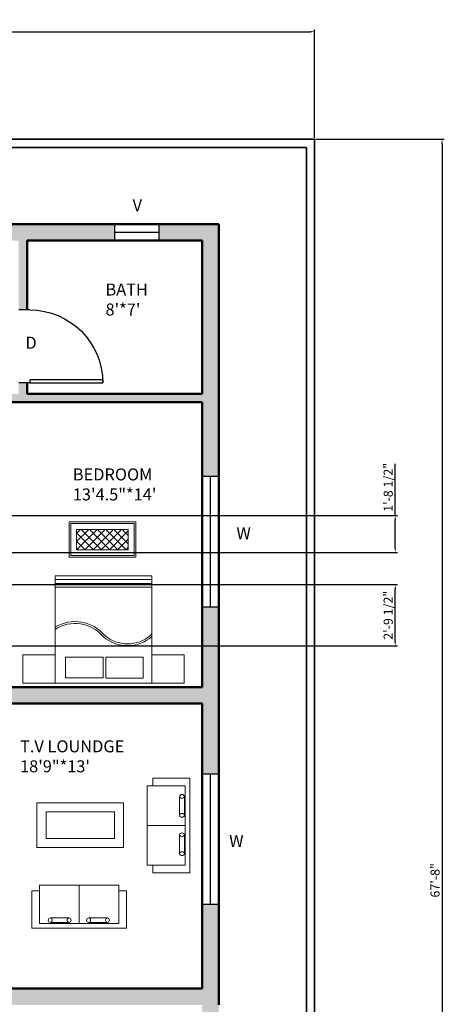
# Model space of a CAD drawing. Units: inches. Extents: x 2101 to 2663, y 1144 to 2069.
# Tile 4 of 4: x 2431 to 2663, y 1530 to 2069. Entities that reach past the tile are written whole.
import ezdxf

# ---------------------------------------------------------------- set-up
doc = ezdxf.new("R2010")
doc.units = ezdxf.units.IN
for name, color, linetype, lineweight in [('A-ANNO-DIMS', 2, 'Continuous', 18), ('A-ANNO-TEXT', 7, 'Continuous', 18), ('A-AREA-IDEN', 7, 'Continuous', 25), ('A-WALL-PATT', 240, 'Continuous', 13), ('C-PROP', 7, 'Continuous', 35), ('door', 52, 'Continuous', 25), ('fur', 142, 'Continuous', 18), ('wall', 240, 'Continuous', 50), ('win', 150, 'Continuous', 25)]:
    doc.layers.add(name, color=color, linetype=linetype, lineweight=lineweight)
doc.styles.get("Standard").update_dxf_attribs({"font": 'arial.ttf'})
doc.dimstyles.new('ISO-25', dxfattribs={"dimtxt": 5, "dimasz": 2.5, "dimexe": 1.25, "dimexo": 0.625, "dimtad": 1, "dimdec": 0, "dimlunit": 4, "dimtxsty": 'Standard', "dimcen": 2.5, "dimadec": 0, "dimazin": 0, "dimtfac": 1, "dimtdec": 0, "dimtmove": 0, "dimatfit": 3, "dimfxl": 1, "dimarcsym": 0})

# ---------------------------------------------------------------- blocks, each defined once
blk = doc.blocks.new('*U2')
for p, q in [((0, 0), (0, -6)), ((40, 0), (40, -6))]:
    blk.add_line(p, q)
blk.add_lwpolyline([(0, 0), (0, 40), (1.75, 40), (1.75, 0)], close=True)
blk.add_arc((0, 0), 40, 0, 90)
blk = doc.blocks.new('*D9')
at = {"layer": 'A-ANNO-DIMS', "color": 0, "lineweight": -2, "transparency": 16777216}
for p, q in [((2112.39, 2004.28), (2112.39, 2063.71)), ((2114.89, 2062.46), (2589.89, 2062.46)), ((2592.39, 2004.28), (2592.39, 2063.71))]:
    blk.add_line(p, q, dxfattribs=at)
at = {"layer": 'A-ANNO-DIMS', "color": 0, "lineweight": 100, "transparency": 16777216}
for points in [[(2114.89, 2062.88), (2114.89, 2062.04), (2112.39, 2062.46)], [(2589.89, 2062.88), (2589.89, 2062.04), (2592.39, 2062.46)]]:
    blk.add_solid(points, dxfattribs=at)
at = {"layer": 'Defpoints', "color": 0, "lineweight": 100, "transparency": 16777216}
for p in [(2592.39, 2062.46), (2112.39, 2003.65), (2592.39, 2003.65)]:
    blk.add_point(p, dxfattribs=at)
at = {"layer": 'A-ANNO-DIMS', "color": 0, "transparency": 16777216, "insert": (2352.39, 2065.64), "char_height": 5, "attachment_point": 5}
blk.add_mtext("40'", dxfattribs=at)
blk = doc.blocks.new('*D10')
at = {"layer": 'A-ANNO-DIMS', "color": 0, "lineweight": -2, "transparency": 16777216}
for p, q in [((2593.02, 2003.65), (2663.42, 2003.65)), ((2662.17, 2001.15), (2662.17, 1194.65)), ((2593.02, 1192.15), (2663.42, 1192.15))]:
    blk.add_line(p, q, dxfattribs=at)
at = {"layer": 'A-ANNO-DIMS', "color": 0, "lineweight": 100, "transparency": 16777216}
for points in [[(2661.75, 2001.15), (2662.59, 2001.15), (2662.17, 2003.65)], [(2661.75, 1194.65), (2662.59, 1194.65), (2662.17, 1192.15)]]:
    blk.add_solid(points, dxfattribs=at)
at = {"layer": 'Defpoints', "color": 0, "lineweight": 100, "transparency": 16777216}
for p in [(2592.39, 2003.65), (2592.39, 1192.15), (2662.17, 1192.15)]:
    blk.add_point(p, dxfattribs=at)
at = {"layer": 'A-ANNO-DIMS', "color": 0, "transparency": 16777216, "insert": (2658.99, 1597.9), "char_height": 5, "attachment_point": 5, "rotation": 90}
blk.add_mtext('67\'-8"', dxfattribs=at)
blk = doc.blocks.new('SOFA-TWO-SEAT')
for p, q in [((-8.65, 21.68), (-8.65, 25.93)), ((-8.65, 25.93), (11.73, 25.93)), ((11.73, 25.93), (11.73, -25.93)), ((-11.73, -0.01), (9.09, -0.01)), ((-8.65, -25.93), (-8.65, -21.7)), ((11.73, -25.93), (-8.65, -25.93))]:
    blk.add_line(p, q)
blk.add_lwpolyline([(9.09, 21.68), (-11.73, 21.68), (-11.73, -21.7), (9.09, -21.7)], close=True)
for points in [[(6.04, 5.2), (6.04, 15.47)], [(8.66, 15.47), (8.66, 5.2)], [(6.04, -15.8), (6.04, -5.54)], [(8.66, -5.54), (8.66, -15.8)]]:
    blk.add_lwpolyline(points)
for centre, radius, start, end in [((7.35, 15.19), 1.34, 11.9211, 168.0789), ((7.35, 15.75), 1.34, 191.8934, 348.1066), ((7.35, 4.81), 1.37, 16.4476, 163.5524), ((7.35, 5.4), 1.33, 188.6987, 351.3013), ((7.35, -5.81), 1.34, 11.9211, 168.0789), ((7.35, -5.26), 1.34, 191.8934, 348.1066), ((7.35, -16.19), 1.37, 16.4476, 163.5524), ((7.35, -15.6), 1.33, 188.6987, 351.3013)]:
    blk.add_arc(centre, radius, start, end)
blk = doc.blocks.new('BED-DOUBLE-WITH-NIGHTSTANDS')
for p, q in [((-26.51, 27.34), (26.51, 27.34)), ((-26.51, 25.17), (26.51, 25.17)), ((-26.51, 23.05), (26.51, 23.05)), ((25.85, -3.2), (26.51, -2.64))]:
    blk.add_line(p, q)
for points in [[(-26.51, -29.4), (26.51, -29.4), (26.51, 29.4), (-26.51, 29.4)], [(-26.51, -29.4), (-44.2, -29.4), (-44.2, -13.89), (-26.51, -13.89)], [(-20.73, -26.56), (-0.14, -26.56), (-0.14, -15.14), (-20.73, -15.14)], [(1.25, -26.65), (21.84, -26.65), (21.84, -15.23), (1.25, -15.23)], [(44.2, -29.4), (26.51, -29.4), (26.51, -13.89), (44.2, -13.89)]]:
    blk.add_lwpolyline(points, close=True)
for centre, radius, start, end in [((-15.51, -16.76), 21.05, 39.687, 121.5045), ((-15.51, -16.76), 20.05, 39.687, 123.273), ((13.21, 11.48), 20.37, 229.27, 310.73), ((13.21, 11.48), 19.37, 229.27, 310.73)]:
    blk.add_arc(centre, radius, start, end)
blk = doc.blocks.new('BEDROOM-BENCH')
h = blk.add_hatch()
h.set_pattern_fill('ANSI37', color=256)
h.set_pattern_definition([(45, (-2254.725, -1882.7455), (-2.245064, 2.245064), []), (135, (-2254.725, -1882.7455), (-2.245064, -2.245064), [])])
h.paths.add_polyline_path([(14.16, 5.58), (-14.16, 5.58), (-14.16, -5.58), (14.16, -5.58)])
for points in [[(-18.29, -9.71), (18.29, -9.71), (18.29, 9.71), (-18.29, 9.71)], [(-17.29, -8.71), (17.29, -8.71), (17.29, 8.71), (-17.29, 8.71)], [(-14.16, -5.58), (14.16, -5.58), (14.16, 5.58), (-14.16, 5.58)]]:
    blk.add_lwpolyline(points, close=True)
blk = doc.blocks.new('*D30')
at = {"layer": 'A-ANNO-DIMS', "color": 0, "lineweight": -2, "transparency": 16777216}
for p, q in [((2146.02, 1759.8), (2637.79, 1759.8)), ((2636.54, 1728.69), (2636.54, 1757.3)), ((2146.02, 1726.19), (2637.79, 1726.19))]:
    blk.add_line(p, q, dxfattribs=at)
at = {"layer": 'A-ANNO-DIMS', "color": 0, "lineweight": 100, "transparency": 16777216}
for points in [[(2636.13, 1757.3), (2636.96, 1757.3), (2636.54, 1759.8)], [(2636.13, 1728.69), (2636.96, 1728.69), (2636.54, 1726.19)]]:
    blk.add_solid(points, dxfattribs=at)
at = {"layer": 'Defpoints', "color": 0, "lineweight": 100, "transparency": 16777216}
for p in [(2145.39, 1759.8), (2636.54, 1759.8), (2145.39, 1726.19)]:
    blk.add_point(p, dxfattribs=at)
at = {"layer": 'A-ANNO-DIMS', "color": 0, "transparency": 16777216, "insert": (2633.33, 1743), "char_height": 5, "attachment_point": 5, "rotation": 90}
blk.add_mtext('2\'-9 1/2"', dxfattribs=at)
blk = doc.blocks.new('*D33')
at = {"layer": 'A-ANNO-DIMS', "color": 0, "lineweight": -2, "transparency": 16777216}
for p, q in [((2636.54, 1797.66), (2636.54, 1825.88)), ((2234.21, 1797.66), (2637.79, 1797.66)), ((2636.54, 1779.87), (2636.54, 1795.16)), ((2234.21, 1777.37), (2637.79, 1777.37))]:
    blk.add_line(p, q, dxfattribs=at)
at = {"layer": 'A-ANNO-DIMS', "color": 0, "lineweight": 100, "transparency": 16777216}
for points in [[(2636.13, 1795.16), (2636.96, 1795.16), (2636.54, 1797.66)], [(2636.13, 1779.87), (2636.96, 1779.87), (2636.54, 1777.37)]]:
    blk.add_solid(points, dxfattribs=at)
at = {"layer": 'Defpoints', "color": 0, "lineweight": 100, "transparency": 16777216}
for p in [(2233.58, 1797.66), (2636.54, 1797.66), (2233.58, 1777.37)]:
    blk.add_point(p, dxfattribs=at)
at = {"layer": 'A-ANNO-DIMS', "color": 0, "transparency": 16777216, "insert": (2633.33, 1813.02), "char_height": 5, "attachment_point": 5, "rotation": 90}
blk.add_mtext('1\'-8 1/2"', dxfattribs=at)

msp = doc.modelspace()

# ---------------------------------------------------------------- hatches: boundary and pattern name
at = {"layer": 'A-WALL-PATT'}
h = msp.add_hatch(color=256, dxfattribs=at)
h.dxf.hatch_style = 1
h.paths.add_polyline_path([(2190.39, 2003.65), (2185.89, 2003.65), (2112.39, 2003.65), (2112.39, 1882.15), (2112.39, 1799.65), (2112.39, 1694.65), (2121.39, 1694.65), (2121.39, 1703.65), (2121.39, 1799.65), (2121.39, 1804.15), (2121.39, 1882.15), (2145.24, 1882.15), (2145.24, 1886.65), (2121.39, 1886.65), (2121.39, 1917.6), (2121.39, 1994.65), (2181.39, 1994.65), (2181.39, 1990.84), (2190.39, 1990.84), (2190.39, 1999.15)])
h.paths.add_polyline_path([(2185.89, 1843.15), (2181.39, 1843.15), (2181.39, 1804.15), (2185.89, 1804.15)], flags=17)
h.paths.add_polyline_path([(2185.89, 1948.15), (2251.48, 1948.15), (2251.48, 1957.15), (2190.39, 1957.15), (2190.39, 1968.84), (2181.39, 1968.84), (2181.39, 1968.14), (2181.39, 1886.65), (2178.82, 1886.65), (2178.82, 1882.15), (2181.39, 1882.15), (2181.39, 1876.17), (2185.89, 1876.17), (2185.89, 1882.15)])
h.paths.add_polyline_path([(2482.89, 1957.15), (2335.68, 1957.15), (2335.68, 1948.15), (2365.89, 1948.15), (2482.89, 1948.15)])
h.paths.add_polyline_path([(2539.89, 1957.15), (2515.98, 1957.15), (2507.18, 1957.15), (2507.18, 1948.15), (2530.89, 1948.15), (2530.89, 1864.15), (2530.89, 1859.65), (2539.89, 1859.65), (2539.89, 1864.15), (2539.89, 1883.02)])
h.paths.add_polyline_path([(2539.89, 1859.65), (2530.89, 1859.65), (2530.89, 1819.07), (2539.89, 1819.07)])
h.paths.add_polyline_path([(2530.89, 1864.15), (2434.89, 1864.15), (2434.89, 1859.65), (2530.89, 1859.65)])
h.paths.add_polyline_path([(2388.94, 1864.15), (2370.39, 1864.15), (2370.39, 1859.65), (2388.94, 1859.65)])
h.paths.add_polyline_path([(2434.89, 1864.15), (2434.89, 1870.19), (2430.39, 1870.19), (2430.39, 1864.15), (2424.15, 1864.15), (2424.15, 1859.65), (2434.89, 1859.65)])
h.paths.add_polyline_path([(2434.89, 1948.15), (2430.39, 1948.15), (2430.39, 1910.19), (2434.89, 1910.19)])
h.paths.add_polyline_path([(2370.39, 1948.15), (2365.89, 1948.15), (2365.89, 1804.15), (2365.89, 1795.15), (2370.39, 1795.15), (2370.39, 1859.65), (2370.39, 1864.15)])
h.paths.add_polyline_path([(2539.89, 1747.47), (2530.89, 1747.47), (2530.89, 1703.65), (2370.39, 1703.65), (2370.39, 1708.72), (2365.89, 1708.72), (2365.89, 1694.65), (2539.89, 1694.65)])
h.paths.add_polyline_path([(2539.89, 1694.65), (2530.89, 1694.65), (2530.89, 1656.23), (2539.89, 1656.23)])
h = msp.add_hatch(color=256, dxfattribs=at)
h.dxf.hatch_style = 1
h.paths.add_polyline_path([(2305.89, 1705.85), (2299.89, 1705.85), (2296.89, 1705.85), (2296.89, 1703.65), (2167.89, 1703.65), (2167.89, 1694.65), (2305.89, 1694.65)])
h.paths.add_polyline_path([(2305.89, 1804.15), (2121.39, 1804.15), (2121.39, 1799.65), (2296.89, 1799.65), (2296.89, 1775.65), (2296.89, 1745.74, -0.01877), (2299.89, 1745.85), (2305.89, 1745.85)])
h.paths.add_polyline_path([(2319.05, 1801.15, -0.01877), (2319.16, 1804.15), (2305.89, 1804.15), (2305.89, 1795.15), (2319.05, 1795.15)])
h.paths.add_polyline_path([(2365.89, 1804.15), (2359.05, 1804.15), (2359.05, 1801.15), (2359.05, 1795.15), (2365.89, 1795.15)])
h.paths.add_polyline_path([(2370.39, 1795.15), (2365.89, 1795.15), (2365.89, 1748.72), (2370.39, 1748.72)])
h.paths.add_polyline_path([(2305.89, 1694.65), (2296.89, 1694.65), (2296.89, 1656.63), (2305.89, 1656.63)])
h.paths.add_polyline_path([(2176.89, 1694.65), (2167.89, 1694.65), (2167.89, 1679.51), (2176.89, 1679.51)])
h.paths.add_polyline_path([(2134.3, 1610.65), (2116.89, 1610.65), (2116.89, 1606.15), (2134.3, 1606.15)])
h.paths.add_polyline_path([(2176.89, 1622.19), (2167.89, 1622.19), (2167.89, 1610.65), (2154.79, 1610.65), (2154.79, 1606.15), (2176.89, 1606.15)])
h.paths.add_polyline_path([(2176.89, 1606.15), (2172.39, 1606.15), (2172.39, 1534.15), (2147.63, 1534.15), (2147.63, 1529.65), (2176.89, 1529.65)])
h.paths.add_polyline_path([(2211.7, 1535.65), (2211.7, 1538.65), (2176.89, 1538.65), (2176.89, 1529.65), (2211.7, 1529.65)])
h.paths.add_polyline_path([(2116.89, 1606.15), (2112.39, 1606.15), (2112.39, 1529.65), (2121.39, 1529.65), (2121.39, 1534.15), (2116.89, 1534.15)])
h.paths.add_polyline_path([(2121.39, 1529.65), (2112.39, 1529.65), (2112.39, 1485), (2121.39, 1485)])
h.paths.add_polyline_path([(2359.39, 1535.65), (2359.39, 1538.65), (2314.89, 1538.65), (2251.59, 1538.65, -0.01877), (2251.7, 1535.65), (2251.7, 1529.65), (2359.39, 1529.65)])
h.paths.add_polyline_path([(2305.89, 1575.46), (2296.89, 1575.46), (2296.89, 1538.65), (2305.89, 1538.65)])
h.paths.add_polyline_path([(2539.89, 1584.63), (2530.89, 1584.63), (2530.89, 1538.65), (2399.28, 1538.65, -0.01877), (2399.39, 1535.65), (2399.39, 1529.65), (2539.89, 1529.65)])
h.paths.add_polyline_path([(2346.39, 1370.88), (2340.39, 1370.88), (2337.39, 1370.88), (2337.39, 1361.65), (2308.27, 1361.65), (2308.27, 1352.65), (2346.39, 1352.65)])
h.paths.add_polyline_path([(2168.45, 1361.65), (2121.39, 1361.65), (2121.39, 1417.42), (2112.39, 1417.42), (2112.39, 1352.65), (2168.45, 1352.65)])
h.paths.add_polyline_path([(2346.39, 1529.65), (2337.39, 1529.65), (2337.39, 1414.47), (2337.39, 1410.77, -0.01877), (2340.39, 1410.88), (2346.39, 1410.88), (2346.39, 1414.47)])
h.paths.add_polyline_path([(2592.39, 1433.97), (2583.39, 1433.97), (2583.39, 1292.97), (2592.39, 1292.97)])
h.paths.add_polyline_path([(2592.39, 1204.95), (2583.39, 1204.95), (2583.39, 1196.65), (2578.02, 1196.65), (2578.02, 1192.15), (2592.39, 1192.15)])
h.paths.add_polyline_path([(2583.39, 1204.95), (2578.02, 1204.95), (2578.02, 1196.65), (2583.39, 1196.65)], flags=17)
h.paths.add_polyline_path([(2382.99, 1204.95), (2368.62, 1204.95), (2368.62, 1196.65), (2382.99, 1196.65)])
h.paths.add_polyline_path([(2382.99, 1196.65), (2368.62, 1196.65), (2368.62, 1192.15), (2382.99, 1192.15)])
h.paths.add_polyline_path([(2490.54, 1433.65), (2490.54, 1424.65), (2539.89, 1424.65), (2539.89, 1433.97), (2539.89, 1529.65), (2530.89, 1529.65), (2530.89, 1433.65)])
h.paths.add_polyline_path([(2438.35, 1424.65), (2438.35, 1433.65), (2400.84, 1433.65), (2400.84, 1424.65)])

# ---------------------------------------------------------------- linework, layer by layer
at = {"layer": 'C-PROP'}
for p, q in [((2185.89, 2003.65), (2515.98, 2003.65)), ((2185.89, 2003.65), (2592.39, 2003.65)), ((2592.39, 2003.65), (2190.39, 2003.65)), ((2592.39, 2003.65), (2592.39, 1893.68)), ((2592.39, 1433.97), (2592.39, 2003.65)), ((2190.39, 1999.15), (2587.89, 1999.15)), ((2190.39, 1999.15), (2587.89, 1999.15)), ((2587.89, 1999.15), (2587.89, 1893.68)), ((2587.89, 1999.15), (2587.89, 1433.97)), ((2587.89, 1893.68), (2587.89, 1448.02)), ((2592.39, 1893.68), (2592.39, 1448.02))]:
    msp.add_line(p, q, dxfattribs=at)
at = {"layer": 'fur'}
for points in [[(2440.34, 1615.79), (2487.74, 1615.79), (2487.74, 1640.33), (2440.34, 1640.33)], [(2445.34, 1620.79), (2482.74, 1620.79), (2482.74, 1635.33), (2445.34, 1635.33)]]:
    msp.add_lwpolyline(points, close=True, dxfattribs=at)
at = {"layer": 'wall'}
for p, q in [((2190.39, 1957.15), (2539.89, 1957.15)), ((2515.98, 1957.15), (2539.89, 1957.15)), ((2539.89, 1957.15), (2539.89, 1876.15)), ((2434.89, 1948.15), (2434.89, 1910.19)), ((2434.89, 1948.15), (2530.89, 1948.15)), ((2434.89, 1948.15), (2515.98, 1948.15)), ((2530.89, 1948.15), (2530.89, 1864.15)), ((2539.89, 1859.65), (2539.89, 1883.02)), ((2434.89, 1870.19), (2434.89, 1864.15)), ((2434.89, 1859.65), (2424.15, 1859.65)), ((2434.89, 1864.15), (2530.89, 1864.15)), ((2434.89, 1859.65), (2530.89, 1859.65)), ((2530.89, 1703.65), (2530.89, 1859.65)), ((2539.89, 1694.65), (2539.89, 1864.15)), ((2370.39, 1703.65), (2530.89, 1703.65)), ((2365.89, 1694.65), (2530.89, 1694.65)), ((2530.89, 1694.65), (2530.89, 1538.65)), ((2530.89, 1694.65), (2530.89, 1538.65)), ((2539.89, 1694.65), (2539.89, 1529.65)), ((2530.89, 1538.65), (2399.28, 1538.65))]:
    msp.add_line(p, q, dxfattribs=at)
at = {"layer": 'win'}
for p, q in [((2482.89, 1952.65), (2507.18, 1952.65)), ((2535.39, 1747.47), (2535.39, 1819.07)), ((2535.39, 1584.63), (2535.39, 1656.23))]:
    msp.add_line(p, q, dxfattribs=at)
for points in [[(2482.89, 1948.15), (2507.18, 1948.15), (2507.18, 1957.15), (2482.89, 1957.15)], [(2530.89, 1819.07), (2539.89, 1819.07), (2539.89, 1747.47), (2530.89, 1747.47)], [(2530.89, 1656.23), (2539.89, 1656.23), (2539.89, 1584.63), (2530.89, 1584.63)]]:
    msp.add_lwpolyline(points, close=True, dxfattribs=at)

# ---------------------------------------------------------------- block references
at = {"layer": 'door', "xscale": -1, "rotation": 270}
msp.add_blockref('*U2', (2436.39, 1870.19), dxfattribs=at)
at = {"layer": 'fur'}
for name, p in [('BEDROOM-BENCH', (2476.21, 1784.45)), ('BED-DOUBLE-WITH-NIGHTSTANDS', (2476.75, 1735.25))]:
    msp.add_blockref(name, p, dxfattribs=at)
at = {"layer": 'fur', "extrusion": (0, 0, -1), "zscale": -1, "rotation": 180}
msp.add_blockref('SOFA-TWO-SEAT', (-2512.41, 1627.95), dxfattribs=at)
at = {"layer": 'fur', "rotation": 270.0000000000029}
msp.add_blockref('SOFA-TWO-SEAT', (2463.49, 1583.43), dxfattribs=at)

# ---------------------------------------------------------------- texts
at = {"layer": 'A-ANNO-TEXT', "char_height": 6.57, "attachment_point": 1}
for s, insert in [('V', (2492.72, 1970.7)), ('D', (2434.05, 1895.46)), ('W', (2549.57, 1791.22)), ('W', (2545.6, 1622.74))]:
    msp.add_mtext_dynamic_manual_height_columns(s, width=76.8305, gutter_width=32.84, heights=[0], dxfattribs=dict(at, insert=insert))
at = {"layer": 'A-AREA-IDEN', "attachment_point": 1}
for s, insert, char_height in [("BATH\\P8'*7'", (2477.87, 1924.62), 6.568), ('BEDROOM\\P13\'4.5"*14\'', (2459.99, 1823.39), 6.5684), ('T.V LOUNDGE\\P18\'9"*13\'', (2431.09, 1674.53), 6.5684)]:
    msp.add_mtext_dynamic_manual_height_columns(s, width=76.8305, gutter_width=32.84, heights=[0], dxfattribs=dict(at, insert=insert, char_height=char_height))

# ---------------------------------------------------------------- dimensions: what is measured, and where the dimension line sits
at = {"layer": 'A-ANNO-DIMS'}
dim = msp.add_linear_dim(base=(2592.39, 2062.46), p1=(2112.39, 2003.65), p2=(2592.39, 2003.65), dimstyle='ISO-25', override={"dimclrd": 0, "dimclre": 0, "dimclrt": 0}, dxfattribs=at)
dim.commit()
dim.dimension.update_dxf_attribs({"geometry": '*D9', "text_midpoint": (2352.39, 2065.64)})
for base, p1, p2, override, picture, middle in [((2662.16897098, 1192.1502194), (2592.39296591, 2003.6502194), (2592.39296591, 1192.1502194), {"dimclrd": 0, "dimclre": 0, "dimclrt": 0}, '*D10', (2658.99110604, 1597.9002194)), ((2636.54, 1797.66), (2233.58, 1777.37), (2233.58, 1797.66), {"dimdec": 1, "dimlfac": 1, "dimrnd": 0, "dimzin": 1, "dimdsep": 46, "dimlunit": 4, "dimfrac": 2}, '*D33', (2633.33, 1813.02)), ((2636.54, 1759.8), (2145.39, 1726.19), (2145.39, 1759.8), {"dimdec": 1, "dimlfac": 1, "dimrnd": 0, "dimzin": 1, "dimdsep": 46, "dimlunit": 4, "dimfrac": 2}, '*D30', (2633.33, 1743))]:
    dim = msp.add_linear_dim(base=base, p1=p1, p2=p2, angle=90, dimstyle='ISO-25', override=override, dxfattribs=at)
    dim.commit()
    dim.dimension.update_dxf_attribs({"geometry": picture, "text_midpoint": middle})

doc.saveas('drawing.dxf')
